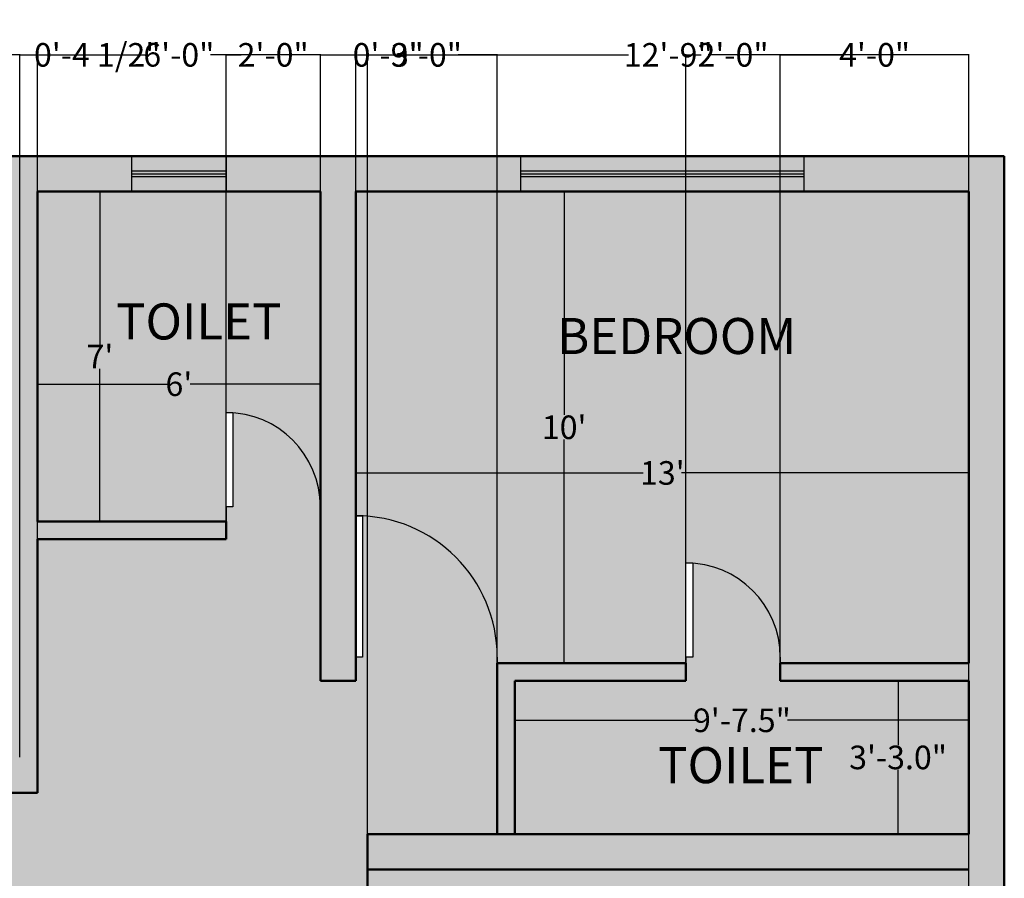
# Model space of a CAD drawing. Units: inches. Extents: x 1379 to 6665, y -118 to 1026.
# Tile 29 of 29: x 6415 to 6665, y 320 to 538. Entities that reach past the tile are written whole.
import ezdxf

# ---------------------------------------------------------------- set-up
doc = ezdxf.new("R2010")
doc.units = ezdxf.units.IN
doc.header["$MEASUREMENT"] = 0
for name, color, linetype, lineweight in [('A-ANNO-DIMS', 2, 'Continuous', 18), ('A-AREA-IDEN', 7, 'Continuous', 25), ('A-DOOR', 1, 'Continuous', 25), ('A-FLOR-PATT', 252, 'Continuous', 13), ('A-GLAZ', 2, 'Continuous', 25), ('A-WALL', 7, 'Continuous', 50), ('A-WALL-PATT', 8, 'Continuous', 13)]:
    doc.layers.add(name, color=color, linetype=linetype, lineweight=lineweight)
doc.styles.get("Standard").update_dxf_attribs({"font": 'arial.ttf'})
doc.dimstyles.get("Standard").update_dxf_attribs({"dimtxt": 6, "dimasz": 0.18, "dimexe": 0.18, "dimexo": 0.0625, "dimgap": 0.09, "dimtad": 0, "dimtih": 1, "dimtoh": 1, "dimdec": 1, "dimzin": 0, "dimdsep": 46, "dimlunit": 3, "dimtxsty": 'Standard', "dimcen": 0.09, "dimclrt": 250, "dimadec": 0, "dimazin": 0, "dimtfac": 1, "dimtdec": 1, "dimtofl": 0, "dimtmove": 0, "dimatfit": 3, "dimfxl": 1, "dimtolj": 1, "dimtzin": 0, "dimarcsym": 0})

# ---------------------------------------------------------------- blocks, each defined once
blk = doc.blocks.new('*U2')
for p, q in [((0, 0), (0, -6)), ((24, 0), (24, -6))]:
    blk.add_line(p, q)
blk.add_lwpolyline([(0, 0), (0, 24), (1.75, 24), (1.75, 0)], close=True)
blk.add_arc((0, 0), 24, 0, 90)
blk = doc.blocks.new('*U3')
for p, q in [((0, 0), (0, -6)), ((36, 0), (36, -6))]:
    blk.add_line(p, q)
blk.add_lwpolyline([(0, 0), (0, 36), (1.75, 36), (1.75, 0)], close=True)
blk.add_arc((0, 0), 36, 0, 90)
blk = doc.blocks.new('*D81')
at = {"layer": 'A-ANNO-DIMS', "color": 0, "lineweight": -2, "transparency": 16777216}
for p, q in [((6419.4, 445.53), (6419.4, 445.42)), ((6419.58, 445.6), (6452.54, 445.6)), ((6491.22, 445.6), (6458.27, 445.6)), ((6491.4, 445.66), (6491.4, 445.78))]:
    blk.add_line(p, q, dxfattribs=at)
at = {"layer": 'A-ANNO-DIMS', "color": 0, "transparency": 16777216}
for points in [[(6419.58, 445.63), (6419.58, 445.57), (6419.4, 445.6)], [(6491.22, 445.63), (6491.22, 445.57), (6491.4, 445.6)]]:
    blk.add_solid(points, dxfattribs=at)
at = {"layer": 'Defpoints', "color": 0, "transparency": 16777216}
for p in [(6419.4, 445.6), (6491.4, 445.6), (6491.4, 445.6)]:
    blk.add_point(p, dxfattribs=at)
at = {"layer": 'A-ANNO-DIMS', "color": 0, "transparency": 16777216, "insert": (6455.4, 445.6), "char_height": 6, "attachment_point": 5}
blk.add_mtext("\\A1;6'", dxfattribs=at)
blk = doc.blocks.new('*D82')
at = {"layer": 'A-ANNO-DIMS', "color": 0, "lineweight": -2, "transparency": 16777216}
for p, q in [((6432.31, 494.64), (6435.49, 494.64)), ((6435.31, 494.46), (6435.31, 455.73)), ((6435.31, 410.82), (6435.31, 449.55)), ((6432.31, 410.64), (6435.49, 410.64))]:
    blk.add_line(p, q, dxfattribs=at)
at = {"layer": 'A-ANNO-DIMS', "color": 0, "transparency": 16777216}
for points in [[(6435.28, 494.46), (6435.34, 494.46), (6435.31, 494.64)], [(6435.28, 410.82), (6435.34, 410.82), (6435.31, 410.64)]]:
    blk.add_solid(points, dxfattribs=at)
at = {"layer": 'Defpoints', "color": 0, "transparency": 16777216}
for p in [(6432.24, 494.64), (6432.24, 410.64), (6435.31, 410.64)]:
    blk.add_point(p, dxfattribs=at)
at = {"layer": 'A-ANNO-DIMS', "color": 0, "transparency": 16777216, "insert": (6435.31, 452.64), "char_height": 6, "attachment_point": 5}
blk.add_mtext("\\A1;7'", dxfattribs=at)
blk = doc.blocks.new('*D83')
at = {"layer": 'A-ANNO-DIMS', "color": 0, "lineweight": -2, "transparency": 16777216}
for p, q in [((6535.1, 494.64), (6553.6, 494.64)), ((6553.42, 494.46), (6553.42, 437.79)), ((6553.42, 374.82), (6553.42, 431.49)), ((6549.51, 374.64), (6553.6, 374.64))]:
    blk.add_line(p, q, dxfattribs=at)
at = {"layer": 'A-ANNO-DIMS', "color": 0, "transparency": 16777216}
for points in [[(6553.39, 494.46), (6553.45, 494.46), (6553.42, 494.64)], [(6553.39, 374.82), (6553.45, 374.82), (6553.42, 374.64)]]:
    blk.add_solid(points, dxfattribs=at)
at = {"layer": 'Defpoints', "color": 0, "transparency": 16777216}
for p in [(6535.04, 494.64), (6549.45, 374.64), (6553.42, 374.64)]:
    blk.add_point(p, dxfattribs=at)
at = {"layer": 'A-ANNO-DIMS', "color": 0, "transparency": 16777216, "insert": (6553.42, 434.64), "char_height": 6, "attachment_point": 5}
blk.add_mtext("\\A1;10'", dxfattribs=at)
blk = doc.blocks.new('*D84')
at = {"layer": 'A-ANNO-DIMS', "color": 0, "lineweight": -2, "transparency": 16777216}
for p, q in [((6500.4, 421.26), (6500.4, 423.2)), ((6500.58, 423.02), (6573.5, 423.02)), ((6656.22, 423.02), (6583.3, 423.02)), ((6656.4, 418.94), (6656.4, 423.2))]:
    blk.add_line(p, q, dxfattribs=at)
at = {"layer": 'A-ANNO-DIMS', "color": 0, "transparency": 16777216}
for points in [[(6500.58, 423.05), (6500.58, 422.99), (6500.4, 423.02)], [(6656.22, 423.05), (6656.22, 422.99), (6656.4, 423.02)]]:
    blk.add_solid(points, dxfattribs=at)
at = {"layer": 'Defpoints', "color": 0, "transparency": 16777216}
for p in [(6500.4, 421.2), (6656.4, 423.02), (6656.4, 418.88)]:
    blk.add_point(p, dxfattribs=at)
at = {"layer": 'A-ANNO-DIMS', "color": 0, "transparency": 16777216, "insert": (6578.4, 423.02), "char_height": 6, "attachment_point": 5}
blk.add_mtext("\\A1;13'", dxfattribs=at)
blk = doc.blocks.new('*D85')
at = {"layer": 'A-ANNO-DIMS', "color": 0, "lineweight": -2, "transparency": 16777216}
for p, q in [((6637.36, 370.14), (6638.56, 370.14)), ((6638.38, 369.96), (6638.38, 353.8)), ((6638.38, 331.32), (6638.38, 347.48)), ((6637.36, 331.14), (6638.56, 331.14))]:
    blk.add_line(p, q, dxfattribs=at)
at = {"layer": 'A-ANNO-DIMS', "color": 0, "transparency": 16777216}
for points in [[(6638.35, 369.96), (6638.41, 369.96), (6638.38, 370.14)], [(6638.35, 331.32), (6638.41, 331.32), (6638.38, 331.14)]]:
    blk.add_solid(points, dxfattribs=at)
at = {"layer": 'Defpoints', "color": 0, "transparency": 16777216}
for p in [(6637.3, 370.14), (6637.3, 331.14), (6638.38, 331.14)]:
    blk.add_point(p, dxfattribs=at)
at = {"layer": 'A-ANNO-DIMS', "color": 0, "transparency": 16777216, "insert": (6638.38, 350.64), "char_height": 6, "attachment_point": 5}
blk.add_mtext('\\A1;3\'-3.0"', dxfattribs=at)
blk = doc.blocks.new('*D86')
at = {"layer": 'A-ANNO-DIMS', "color": 0, "lineweight": -2, "transparency": 16777216}
for p, q in [((6540.9, 354.74), (6540.9, 360.27)), ((6541.08, 360.09), (6587.09, 360.09)), ((6656.22, 360.09), (6610.21, 360.09)), ((6656.4, 350.7), (6656.4, 360.27))]:
    blk.add_line(p, q, dxfattribs=at)
at = {"layer": 'A-ANNO-DIMS', "color": 0, "transparency": 16777216}
for points in [[(6541.08, 360.12), (6541.08, 360.06), (6540.9, 360.09)], [(6656.22, 360.12), (6656.22, 360.06), (6656.4, 360.09)]]:
    blk.add_solid(points, dxfattribs=at)
at = {"layer": 'Defpoints', "color": 0, "transparency": 16777216}
for p in [(6656.4, 360.09), (6540.9, 354.68), (6656.4, 350.64)]:
    blk.add_point(p, dxfattribs=at)
at = {"layer": 'A-ANNO-DIMS', "color": 0, "transparency": 16777216, "insert": (6598.65, 360.09), "char_height": 6, "attachment_point": 5}
blk.add_mtext('\\A1;9\'-7.5"', dxfattribs=at)
blk = doc.blocks.new('WIN-1800')
for p, q in [((0, 0.73), (72, 0.73)), ((0, 0), (72, 0))]:
    blk.add_line(p, q)
blk = doc.blocks.new('WIN-600')
for p, q in [((0, 24), (0, 0)), ((0.73, 24), (0.73, 0))]:
    blk.add_line(p, q)
blk = doc.blocks.new('*D139')
at = {"layer": 'A-ANNO-DIMS', "color": 0, "lineweight": -2, "transparency": 16777216}
for p, q in [((6414.9, 494.7), (6414.9, 529.57)), ((6415.08, 529.39), (6419.22, 529.39)), ((6419.4, 494.7), (6419.4, 529.57)), ((6419.4, 529.39), (6419.58, 529.39))]:
    blk.add_line(p, q, dxfattribs=at)
at = {"layer": 'A-ANNO-DIMS', "color": 0, "transparency": 16777216}
for points in [[(6415.08, 529.42), (6415.08, 529.36), (6414.9, 529.39)], [(6419.22, 529.42), (6419.22, 529.36), (6419.4, 529.39)]]:
    blk.add_solid(points, dxfattribs=at)
at = {"layer": 'Defpoints', "color": 0, "transparency": 16777216}
for p in [(6419.4, 529.39), (6414.9, 494.64), (6419.4, 494.64)]:
    blk.add_point(p, dxfattribs=at)
at = {"layer": 'A-ANNO-DIMS', "color": 250, "transparency": 16777216, "insert": (6434.64, 529.39), "char_height": 6, "attachment_point": 5}
blk.add_mtext('\\A1;0\'-4 1/2"', dxfattribs=at)
blk = doc.blocks.new('*D140')
at = {"layer": 'A-ANNO-DIMS', "color": 0, "lineweight": -2, "transparency": 16777216}
for p, q in [((6491.4, 494.7), (6491.4, 529.57)), ((6491.58, 529.39), (6500.22, 529.39)), ((6500.4, 494.7), (6500.4, 529.57)), ((6500.4, 529.39), (6500.58, 529.39))]:
    blk.add_line(p, q, dxfattribs=at)
at = {"layer": 'A-ANNO-DIMS', "color": 0, "transparency": 16777216}
for points in [[(6491.58, 529.42), (6491.58, 529.36), (6491.4, 529.39)], [(6500.22, 529.42), (6500.22, 529.36), (6500.4, 529.39)]]:
    blk.add_solid(points, dxfattribs=at)
at = {"layer": 'Defpoints', "color": 0, "transparency": 16777216}
for p in [(6500.4, 529.39), (6491.4, 494.64), (6500.4, 494.64)]:
    blk.add_point(p, dxfattribs=at)
at = {"layer": 'A-ANNO-DIMS', "color": 250, "transparency": 16777216, "insert": (6508.65, 529.39), "char_height": 6, "attachment_point": 5}
blk.add_mtext('\\A1;0\'-9"', dxfattribs=at)
blk = doc.blocks.new('*D141')
at = {"layer": 'A-ANNO-DIMS', "color": 0, "lineweight": -2, "transparency": 16777216}
for p, q in [((6419.4, 406.2), (6419.4, 529.57)), ((6419.58, 529.39), (6447.32, 529.39)), ((6491.22, 529.39), (6463.48, 529.39)), ((6491.4, 370.2), (6491.4, 529.57))]:
    blk.add_line(p, q, dxfattribs=at)
at = {"layer": 'A-ANNO-DIMS', "color": 0, "transparency": 16777216}
for points in [[(6419.58, 529.42), (6419.58, 529.36), (6419.4, 529.39)], [(6491.22, 529.42), (6491.22, 529.36), (6491.4, 529.39)]]:
    blk.add_solid(points, dxfattribs=at)
at = {"layer": 'Defpoints', "color": 0, "transparency": 16777216}
for p in [(6491.4, 529.39), (6419.4, 406.14), (6491.4, 370.14)]:
    blk.add_point(p, dxfattribs=at)
at = {"layer": 'A-ANNO-DIMS', "color": 250, "transparency": 16777216, "insert": (6455.4, 529.39), "char_height": 6, "attachment_point": 5}
blk.add_mtext('\\A1;6\'-0"', dxfattribs=at)
blk = doc.blocks.new('*D142')
at = {"layer": 'A-ANNO-DIMS', "color": 0, "lineweight": -2, "transparency": 16777216}
for p, q in [((6503.4, 317.7), (6503.4, 529.57)), ((6503.58, 529.39), (6569.79, 529.39)), ((6656.22, 529.39), (6590.02, 529.39)), ((6656.4, 317.7), (6656.4, 529.57))]:
    blk.add_line(p, q, dxfattribs=at)
at = {"layer": 'A-ANNO-DIMS', "color": 0, "transparency": 16777216}
for points in [[(6503.58, 529.42), (6503.58, 529.36), (6503.4, 529.39)], [(6656.22, 529.42), (6656.22, 529.36), (6656.4, 529.39)]]:
    blk.add_solid(points, dxfattribs=at)
at = {"layer": 'Defpoints', "color": 0, "transparency": 16777216}
for p in [(6656.4, 529.39), (6503.4, 317.64), (6656.4, 317.64)]:
    blk.add_point(p, dxfattribs=at)
at = {"layer": 'A-ANNO-DIMS', "color": 250, "transparency": 16777216, "insert": (6579.9, 529.39), "char_height": 6, "attachment_point": 5}
blk.add_mtext('\\A1;12\'-9"', dxfattribs=at)
blk = doc.blocks.new('*D143')
at = {"layer": 'A-ANNO-DIMS', "color": 0, "lineweight": -2, "transparency": 16777216}
for p, q in [((6384.78, 350.7), (6384.78, 529.57)), ((6384.96, 529.39), (6391.72, 529.39)), ((6414.72, 529.39), (6407.96, 529.39)), ((6414.9, 350.7), (6414.9, 529.57))]:
    blk.add_line(p, q, dxfattribs=at)
at = {"layer": 'A-ANNO-DIMS', "color": 0, "transparency": 16777216}
for points in [[(6384.96, 529.42), (6384.96, 529.36), (6384.78, 529.39)], [(6414.72, 529.42), (6414.72, 529.36), (6414.9, 529.39)]]:
    blk.add_solid(points, dxfattribs=at)
at = {"layer": 'Defpoints', "color": 0, "transparency": 16777216}
for p in [(6414.9, 529.39), (6384.78, 350.64), (6414.9, 350.64)]:
    blk.add_point(p, dxfattribs=at)
at = {"layer": 'A-ANNO-DIMS', "color": 250, "transparency": 16777216, "insert": (6399.84, 529.39), "char_height": 6, "attachment_point": 5}
blk.add_mtext('\\A1;2\'-6"', dxfattribs=at)
blk = doc.blocks.new('*D146')
at = {"layer": 'A-ANNO-DIMS', "color": 0, "lineweight": -2, "transparency": 16777216}
for p, q in [((6467.4, 410.7), (6467.4, 529.57)), ((6467.58, 529.39), (6471.29, 529.39)), ((6491.22, 529.39), (6487.52, 529.39)), ((6491.4, 410.7), (6491.4, 529.57))]:
    blk.add_line(p, q, dxfattribs=at)
at = {"layer": 'A-ANNO-DIMS', "color": 0, "transparency": 16777216}
for points in [[(6467.58, 529.42), (6467.58, 529.36), (6467.4, 529.39)], [(6491.22, 529.42), (6491.22, 529.36), (6491.4, 529.39)]]:
    blk.add_solid(points, dxfattribs=at)
at = {"layer": 'Defpoints', "color": 0, "transparency": 16777216}
for p in [(6491.4, 529.39), (6467.4, 410.64), (6491.4, 410.64)]:
    blk.add_point(p, dxfattribs=at)
at = {"layer": 'A-ANNO-DIMS', "color": 250, "transparency": 16777216, "insert": (6479.4, 529.39), "char_height": 6, "attachment_point": 5}
blk.add_mtext('\\A1;2\'-0"', dxfattribs=at)
blk = doc.blocks.new('*D148')
at = {"layer": 'A-ANNO-DIMS', "color": 0, "lineweight": -2, "transparency": 16777216}
for p, q in [((6500.4, 374.7), (6500.4, 529.57)), ((6500.58, 529.39), (6510.34, 529.39)), ((6536.22, 529.39), (6526.46, 529.39)), ((6536.4, 374.7), (6536.4, 529.57))]:
    blk.add_line(p, q, dxfattribs=at)
at = {"layer": 'A-ANNO-DIMS', "color": 0, "transparency": 16777216}
for points in [[(6500.58, 529.42), (6500.58, 529.36), (6500.4, 529.39)], [(6536.22, 529.42), (6536.22, 529.36), (6536.4, 529.39)]]:
    blk.add_solid(points, dxfattribs=at)
at = {"layer": 'Defpoints', "color": 0, "transparency": 16777216}
for p in [(6536.4, 529.39), (6500.4, 374.64), (6536.4, 374.64)]:
    blk.add_point(p, dxfattribs=at)
at = {"layer": 'A-ANNO-DIMS', "color": 250, "transparency": 16777216, "insert": (6518.4, 529.39), "char_height": 6, "attachment_point": 5}
blk.add_mtext('\\A1;3\'-0"', dxfattribs=at)
blk = doc.blocks.new('*D150')
at = {"layer": 'A-ANNO-DIMS', "color": 0, "lineweight": -2, "transparency": 16777216}
for p, q in [((6584.4, 374.7), (6584.4, 529.57)), ((6584.58, 529.39), (6588.29, 529.39)), ((6608.22, 529.39), (6604.52, 529.39)), ((6608.4, 374.7), (6608.4, 529.57))]:
    blk.add_line(p, q, dxfattribs=at)
at = {"layer": 'A-ANNO-DIMS', "color": 0, "transparency": 16777216}
for points in [[(6584.58, 529.42), (6584.58, 529.36), (6584.4, 529.39)], [(6608.22, 529.42), (6608.22, 529.36), (6608.4, 529.39)]]:
    blk.add_solid(points, dxfattribs=at)
at = {"layer": 'Defpoints', "color": 0, "transparency": 16777216}
for p in [(6608.4, 529.39), (6584.4, 374.64), (6608.4, 374.64)]:
    blk.add_point(p, dxfattribs=at)
at = {"layer": 'A-ANNO-DIMS', "color": 250, "transparency": 16777216, "insert": (6596.4, 529.39), "char_height": 6, "attachment_point": 5}
blk.add_mtext('\\A1;2\'-0"', dxfattribs=at)
blk = doc.blocks.new('*D151')
at = {"layer": 'A-ANNO-DIMS', "color": 0, "lineweight": -2, "transparency": 16777216}
for p, q in [((6608.4, 374.7), (6608.4, 529.57)), ((6608.58, 529.39), (6624.22, 529.39)), ((6656.22, 529.39), (6640.59, 529.39)), ((6656.4, 374.7), (6656.4, 529.57))]:
    blk.add_line(p, q, dxfattribs=at)
at = {"layer": 'A-ANNO-DIMS', "color": 0, "transparency": 16777216}
for points in [[(6608.58, 529.42), (6608.58, 529.36), (6608.4, 529.39)], [(6656.22, 529.42), (6656.22, 529.36), (6656.4, 529.39)]]:
    blk.add_solid(points, dxfattribs=at)
at = {"layer": 'Defpoints', "color": 0, "transparency": 16777216}
for p in [(6656.4, 529.39), (6608.4, 374.64), (6656.4, 374.64)]:
    blk.add_point(p, dxfattribs=at)
at = {"layer": 'A-ANNO-DIMS', "color": 250, "transparency": 16777216, "insert": (6632.4, 529.39), "char_height": 6, "attachment_point": 5}
blk.add_mtext('\\A1;4\'-0"', dxfattribs=at)

msp = doc.modelspace()

# ---------------------------------------------------------------- hatches: boundary and pattern name
at = {"layer": 'A-FLOR-PATT', "transparency": 33554590}
h = msp.add_hatch(color=256, dxfattribs=at)
h.dxf.hatch_style = 1
h.paths.add_polyline_path([(6176.4, 382.14), (6176.4, 494.64), (6255.9, 494.64), (6255.9, 503.64), (6167.4, 503.64), (6167.4, 391.14), (6167.4, 323.64), (6176.4, 323.64), (6176.4, 341.64), (6348.9, 341.64), (6348.9, 350.64), (6176.4, 350.64)])
h.paths.add_polyline_path([(6348.9, 233.64), (6176.4, 233.64), (6176.4, 251.64), (6167.4, 251.64), (6167.4, 71.64), (6246.02, 71.64), (6246.02, 80.64), (6176.4, 80.64), (6176.4, 224.64), (6348.9, 224.64)])
h.paths.add_polyline_path([(6443.4, 80.64), (6419.4, 80.64), (6419.4, 164.64), (6467.4, 164.64), (6467.4, 169.14), (6419.4, 169.14), (6419.4, 224.64), (6419.4, 233.64), (6384.87, 233.64), (6384.9, 224.64), (6414.9, 224.64), (6414.9, 80.64), (6318.02, 80.64), (6318.02, 71.64), (6443.4, 71.64)])
h.paths.add_polyline_path([(6552.9, 80.64), (6500.4, 80.64), (6500.4, 169.14), (6491.4, 169.14), (6491.4, 164.64), (6491.4, 80.64), (6467.4, 80.64), (6467.4, 71.64), (6503.4, 71.64), (6552.9, 71.64)])
h.paths.add_polyline_path([(6665.4, 188.64), (6656.4, 188.64), (6656.4, 176.64), (6626.4, 176.64), (6626.4, 172.14), (6656.4, 172.14), (6656.4, 80.64), (6624.9, 80.64), (6624.9, 71.64), (6665.4, 71.64)])
h.paths.add_polyline_path([(6665.4, 503.64), (6614.4, 503.64), (6614.4, 494.64), (6656.4, 494.64), (6656.4, 374.64), (6608.4, 374.64), (6608.4, 370.14), (6656.4, 370.14), (6656.4, 331.14), (6512.4, 331.14), (6503.4, 331.14), (6503.4, 322.14), (6503.4, 317.64), (6656.4, 317.64), (6656.4, 233.64), (6503.4, 233.64), (6455.4, 233.64), (6455.4, 224.64), (6503.4, 224.64), (6567.9, 224.64), (6567.9, 176.64), (6540.4, 176.64), (6540.4, 172.14), (6567.9, 172.14), (6602.4, 172.14), (6602.4, 176.64), (6572.4, 176.64), (6572.4, 224.64), (6656.4, 224.64), (6656.4, 212.64), (6665.4, 212.64)])
h.paths.add_polyline_path([(6584.4, 374.64), (6536.4, 374.64), (6536.4, 370.14), (6536.4, 331.14), (6540.9, 331.14), (6540.9, 370.14), (6584.4, 370.14)], flags=17)
h.paths.add_polyline_path([(6500.4, 494.64), (6542.4, 494.64), (6542.4, 503.64), (6467.4, 503.64), (6467.4, 494.64), (6491.4, 494.64), (6491.4, 370.14), (6500.4, 370.14), (6500.4, 374.64)], flags=17)
h.paths.add_polyline_path([(6443.4, 503.64), (6407.4, 503.64), (6327.9, 503.64), (6327.9, 494.64), (6407.4, 494.64), (6414.9, 494.64), (6414.9, 350.64), (6384.78, 350.64), (6384.9, 341.64), (6419.4, 341.64), (6419.4, 406.14), (6467.4, 406.14), (6467.4, 410.64), (6419.4, 410.64), (6419.4, 494.64), (6443.4, 494.64)])
at = {"layer": 'A-WALL-PATT', "transparency": 33554590}
h = msp.add_hatch(color=256, dxfattribs=at)
h.dxf.hatch_style = 1
h.paths.add_polyline_path([(6467.4, 503.64), (6443.4, 503.64), (6443.4, 499.87), (6467.4, 499.87)])
h.paths.add_polyline_path([(6467.4, 498.41), (6443.4, 498.41), (6443.4, 494.64), (6467.4, 494.64)])
h.paths.add_polyline_path([(6467.4, 499.14), (6443.4, 499.14), (6443.4, 498.41), (6467.4, 498.41)])
h.paths.add_polyline_path([(6467.4, 499.87), (6443.4, 499.87), (6443.4, 499.14), (6467.4, 499.14)])
at = {"layer": 'A-WALL-PATT', "transparency": 33554564}
h = msp.add_hatch(color=256, dxfattribs=at)
h.dxf.hatch_style = 1
h.paths.add_polyline_path([(6614.4, 503.64), (6542.4, 503.64), (6542.4, 499.87), (6614.4, 499.87)])
h.paths.add_polyline_path([(6614.4, 499.14), (6542.4, 499.14), (6542.4, 498.41), (6614.4, 498.41)])
h.paths.add_polyline_path([(6614.4, 499.87), (6542.4, 499.87), (6542.4, 499.14), (6614.4, 499.14)])
h.paths.add_polyline_path([(6614.4, 498.41), (6542.4, 498.41), (6542.4, 494.64), (6614.4, 494.64)])
at = {"layer": 'A-WALL-PATT', "transparency": 33554590}
h = msp.add_hatch(color=256, dxfattribs=at)
h.dxf.hatch_style = 1
h.paths.add_polyline_path([(6414.9, 494.64), (6176.4, 494.64), (6176.4, 382.14), (6176.4, 350.64), (6348.9, 350.64), (6348.9, 383.64), (6350.65, 383.64), (6350.65, 383.6, -0.376042), (6384.78, 350.64), (6414.9, 350.64)])
h.paths.add_polyline_path([(6503.4, 317.64), (6503.4, 322.14), (6503.4, 331.14), (6512.4, 331.14), (6536.4, 331.14), (6536.4, 370.14), (6536.4, 376.14, 0.400041), (6502.15, 412.1), (6502.15, 376.14), (6500.4, 376.14), (6500.4, 370.14), (6491.4, 370.14), (6491.4, 414.39, 0.392996), (6469.15, 438.33), (6469.15, 414.39), (6467.4, 414.39), (6467.4, 408.39), (6467.4, 406.14), (6419.4, 406.14), (6419.4, 341.64), (6384.9, 341.64), (6384.78, 350.64, 0.376042), (6350.65, 383.6), (6350.65, 347.64), (6348.9, 347.64), (6348.9, 341.64), (6176.4, 341.64), (6176.4, 233.64), (6348.9, 233.64), (6348.9, 266.64), (6350.65, 266.64), (6350.65, 266.6, -0.376042), (6384.78, 233.64), (6419.4, 233.64), (6419.4, 224.64), (6419.4, 169.14), (6467.4, 169.14), (6467.4, 172.89), (6467.4, 196.89), (6469.15, 196.89), (6469.15, 196.83, -0.392996), (6491.4, 172.89), (6491.4, 169.14), (6500.4, 169.14), (6500.4, 175.14), (6500.4, 215.14), (6502.15, 215.14), (6502.15, 215.1, -0.390605), (6540.37, 176.64), (6567.9, 176.64), (6567.9, 224.64), (6500.4, 224.64), (6455.4, 224.64), (6455.4, 233.64), (6503.4, 233.64), (6503.4, 275.64)])
h.paths.add_polyline_path([(6491.4, 494.64), (6419.4, 494.64), (6419.4, 410.64), (6467.4, 410.64), (6467.4, 414.39), (6467.4, 438.39), (6469.15, 438.39), (6469.15, 438.33, -0.392996), (6491.4, 414.39)])
h.paths.add_polyline_path([(6656.4, 494.64), (6500.4, 494.64), (6500.4, 412.14), (6502.15, 412.14), (6502.15, 412.1, -0.400041), (6536.4, 376.14), (6536.4, 374.64), (6584.4, 374.64), (6584.4, 376.14), (6584.4, 400.14), (6586.15, 400.14), (6586.15, 400.08, -0.392996), (6608.4, 376.14), (6608.4, 374.64), (6656.4, 374.64)])
h.paths.add_polyline_path([(6414.9, 224.64), (6384.9, 224.64), (6384.87, 233.64), (6384.78, 233.64, 0.376042), (6350.65, 266.6), (6350.65, 266.64), (6348.9, 266.64), (6348.9, 233.64), (6348.9, 224.64), (6176.4, 224.64), (6176.4, 80.64), (6414.9, 80.64)])
h.paths.add_polyline_path([(6491.4, 164.64), (6491.4, 169.14), (6491.4, 172.89, 0.392996), (6469.15, 196.83), (6469.15, 172.89), (6467.4, 172.89), (6467.4, 169.14), (6467.4, 166.89), (6467.4, 164.64), (6419.4, 164.64), (6419.4, 80.64), (6491.4, 80.64)])
h.paths.add_polyline_path([(6656.4, 172.14), (6626.4, 172.14), (6626.4, 178.14, 0.392996), (6604.15, 202.08), (6604.15, 178.14), (6602.4, 178.14), (6602.4, 172.14), (6567.9, 172.14), (6540.4, 172.14), (6540.4, 175.14, 0.401453), (6502.15, 215.1), (6502.15, 175.14), (6500.4, 175.14), (6500.4, 169.14), (6500.4, 80.64), (6503.4, 80.64), (6656.4, 80.64)])
h.paths.add_polyline_path([(6656.4, 224.64), (6572.4, 224.64), (6572.4, 176.64), (6602.4, 176.64), (6602.4, 178.14), (6602.4, 202.14), (6604.15, 202.14), (6604.15, 202.08, -0.392996), (6626.4, 178.14), (6626.4, 176.64), (6656.4, 176.64)])
h.paths.add_polyline_path([(6656.4, 370.14), (6608.4, 370.14), (6608.4, 376.14, 0.392996), (6586.15, 400.08), (6586.15, 376.14), (6584.4, 376.14), (6584.4, 374.64), (6584.4, 370.14), (6540.9, 370.14), (6540.9, 331.14), (6656.4, 331.14)])
h.paths.add_polyline_path([(6259.03, 431.04), (6329.97, 431.04), (6329.97, 445.28), (6259.03, 445.28)], flags=24)
h.paths.add_polyline_path([(6256.77, 281.02), (6365.45, 281.02), (6365.45, 295.25), (6256.77, 295.25)], flags=24)
h.paths.add_polyline_path([(6437.04, 454.45), (6486.63, 454.45), (6486.63, 468.69), (6437.04, 468.69)], flags=24)
h.paths.add_polyline_path([(6549.24, 450.74), (6620.18, 450.74), (6620.18, 464.98), (6549.24, 464.98)], flags=24)
h.paths.add_polyline_path([(6259.03, 146.52), (6329.97, 146.52), (6329.97, 160.75), (6259.03, 160.75)], flags=24)
h.paths.add_polyline_path([(6431.31, 122.15), (6480.89, 122.15), (6480.89, 136.39), (6431.31, 136.39)], flags=24)
h.paths.add_polyline_path([(6550.53, 122.44), (6621.47, 122.44), (6621.47, 136.68), (6550.53, 136.68)], flags=24)
h.paths.add_polyline_path([(6590.78, 206.76), (6640.36, 206.76), (6640.36, 221), (6590.78, 221)], flags=24)
h.paths.add_polyline_path([(6574.95, 341.57), (6624.53, 341.57), (6624.53, 355.8), (6574.95, 355.8)], flags=24)

# ---------------------------------------------------------------- linework, layer by layer
at = {"layer": 'A-GLAZ'}
for p, q in [((6443.4, 498.41), (6467.4, 498.41)), ((6542.4, 498.41), (6614.4, 498.41))]:
    msp.add_line(p, q, dxfattribs=at)
for points in [[(6443.4, 503.64), (6467.4, 503.64), (6467.4, 494.64), (6443.4, 494.64)], [(6542.4, 503.64), (6614.4, 503.64), (6614.4, 494.64), (6542.4, 494.64)]]:
    msp.add_lwpolyline(points, close=True, dxfattribs=at)
at = {"layer": 'A-WALL'}
for p, q in [((6665.4, 503.64), (6407.4, 503.64)), ((6665.4, 503.64), (6665.4, 71.64)), ((6491.4, 494.64), (6419.4, 494.64)), ((6419.4, 410.64), (6419.4, 494.64)), ((6491.4, 370.14), (6491.4, 494.64)), ((6656.4, 494.64), (6500.4, 494.64)), ((6500.4, 374.64), (6500.4, 494.64)), ((6656.4, 494.64), (6656.4, 374.64)), ((6467.4, 410.64), (6419.4, 410.64)), ((6467.4, 410.64), (6467.4, 406.14)), ((6491.4, 410.64), (6491.4, 406.14)), ((6419.4, 341.64), (6419.4, 406.14)), ((6467.4, 406.14), (6419.4, 406.14)), ((6500.4, 374.64), (6500.4, 370.14)), ((6584.4, 374.64), (6536.4, 374.64)), ((6536.4, 374.64), (6536.4, 370.14)), ((6584.4, 370.14), (6584.4, 374.64)), ((6656.4, 374.64), (6608.4, 374.64)), ((6608.4, 370.14), (6608.4, 374.64)), ((6500.4, 370.14), (6491.4, 370.14)), ((6536.4, 370.14), (6536.4, 331.14)), ((6584.4, 370.14), (6540.9, 370.14)), ((6540.9, 370.14), (6540.9, 331.14)), ((6656.4, 370.14), (6608.4, 370.14)), ((6656.4, 370.14), (6656.4, 331.14)), ((6419.4, 341.64), (6384.9, 341.64)), ((6503.4, 322.14), (6503.4, 331.14)), ((6503.4, 331.14), (6512.4, 331.14)), ((6512.4, 331.14), (6656.4, 331.14)), ((6503.4, 322.14), (6503.4, 317.64)), ((6512.4, 322.14), (6503.4, 322.14)), ((6512.4, 322.14), (6656.4, 322.14))]:
    msp.add_line(p, q, dxfattribs=at)

# ---------------------------------------------------------------- block references
at = {"layer": 'A-DOOR'}
for name, p in [('*U2', (6467.4, 414.39)), ('*U3', (6500.4, 376.14)), ('*U2', (6584.4, 376.14))]:
    msp.add_blockref(name, p, dxfattribs=at)
at = {"layer": 'A-GLAZ', "rotation": 90.00000000000134}
msp.add_blockref('WIN-600', (6467.4, 499.14), dxfattribs=at)
at = {"layer": 'A-GLAZ'}
msp.add_blockref('WIN-1800', (6542.4, 499.14), dxfattribs=at)

# ---------------------------------------------------------------- texts
at = {"layer": 'A-AREA-IDEN'}
for s, p in [('TOILET', (6439.42, 456.98)), ('BEDROOM', (6551.61, 453.27)), ('TOILET', (6577.32, 344.09))]:
    msp.add_text(s, height=9.17, dxfattribs=at).set_placement(p)

# ---------------------------------------------------------------- dimensions: what is measured, and where the dimension line sits
at = {"layer": 'A-ANNO-DIMS'}
for base, p1, p2, override, picture, middle in [((6419.4, 529.39), (6414.9, 494.64), (6419.4, 494.64), {"dimdec": 1, "dimlfac": 1, "dimrnd": 0, "dimzin": 1, "dimdsep": 46, "dimlunit": 4, "dimfrac": 2}, '*D139', (6434.64, 529.39)), ((6414.9, 529.39), (6384.78, 350.64), (6414.9, 350.64), {"dimdec": 1, "dimlfac": 1, "dimrnd": 0, "dimzin": 1, "dimdsep": 46, "dimlunit": 4, "dimfrac": 2}, '*D143', (6399.84, 529.39)), ((6491.4, 529.39), (6419.4, 406.14), (6491.4, 370.14), {"dimdec": 1, "dimlfac": 1, "dimrnd": 0, "dimzin": 1, "dimdsep": 46, "dimlunit": 4, "dimfrac": 2}, '*D141', (6455.4, 529.39)), ((6491.4, 529.39), (6467.4, 410.64), (6491.4, 410.64), {"dimdec": 1, "dimlfac": 1, "dimrnd": 0, "dimzin": 1, "dimdsep": 46, "dimlunit": 4, "dimfrac": 2}, '*D146', (6479.4, 529.39)), ((6500.4, 529.39), (6491.4, 494.64), (6500.4, 494.64), {"dimdec": 1, "dimlfac": 1, "dimrnd": 0, "dimzin": 1, "dimdsep": 46, "dimlunit": 4, "dimfrac": 2}, '*D140', (6508.65, 529.39)), ((6536.4, 529.39), (6500.4, 374.64), (6536.4, 374.64), {"dimdec": 1, "dimlfac": 1, "dimrnd": 0, "dimzin": 1, "dimdsep": 46, "dimlunit": 4, "dimfrac": 2}, '*D148', (6518.4, 529.39)), ((6656.4, 529.39), (6503.4, 317.64), (6656.4, 317.64), {"dimdec": 1, "dimlfac": 1, "dimrnd": 0, "dimzin": 1, "dimdsep": 46, "dimlunit": 4, "dimfrac": 2}, '*D142', (6579.9, 529.39)), ((6608.4, 529.39), (6584.4, 374.64), (6608.4, 374.64), {"dimdec": 1, "dimlfac": 1, "dimrnd": 0, "dimzin": 1, "dimdsep": 46, "dimlunit": 4, "dimfrac": 2}, '*D150', (6596.4, 529.39)), ((6656.4, 529.39), (6608.4, 374.64), (6656.4, 374.64), {"dimdec": 1, "dimlfac": 1, "dimrnd": 0, "dimzin": 1, "dimdsep": 46, "dimlunit": 4, "dimfrac": 2}, '*D151', (6632.4, 529.39)), ((6491.4, 445.6), (6419.4, 445.6), (6491.4, 445.6), {"dimclrd": 0, "dimclre": 0, "dimclrt": 0}, '*D81', (6455.4, 445.6)), ((6656.4, 423.02), (6500.4, 421.2), (6656.4, 418.88), {"dimclrd": 0, "dimclre": 0, "dimclrt": 0}, '*D84', (6578.4, 423.02)), ((6656.4, 360.09), (6540.9, 354.68), (6656.4, 350.64), {"dimclrd": 0, "dimclre": 0, "dimclrt": 0}, '*D86', (6598.65, 360.09))]:
    dim = msp.add_linear_dim(base=base, p1=p1, p2=p2, dimstyle='Standard', override=override, dxfattribs=at)
    dim.commit()
    dim.dimension.update_dxf_attribs({"geometry": picture, "text_midpoint": middle})
for base, p1, p2, picture, middle in [((6435.31, 410.64), (6432.24, 494.64), (6432.24, 410.64), '*D82', (6435.31, 452.64)), ((6553.42, 374.64), (6535.04, 494.64), (6549.45, 374.64), '*D83', (6553.42, 434.64)), ((6638.38, 331.14), (6637.3, 370.14), (6637.3, 331.14), '*D85', (6638.38, 350.64))]:
    dim = msp.add_linear_dim(base=base, p1=p1, p2=p2, angle=90, dimstyle='Standard', override={"dimclrd": 0, "dimclre": 0, "dimclrt": 0}, dxfattribs=at)
    dim.commit()
    dim.dimension.update_dxf_attribs({"geometry": picture, "text_midpoint": middle})

doc.saveas('drawing.dxf')
